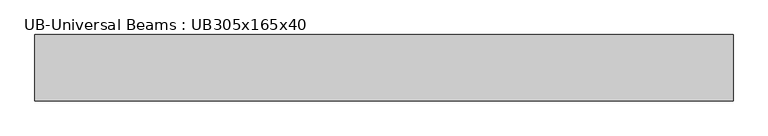
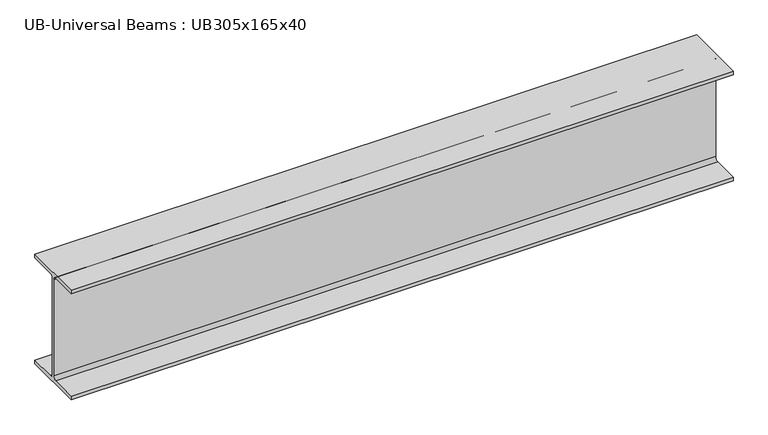
"""IFC4 building model written with IfcOpenShell, lengths in millimetres: beam geometry, UB-Universal Beams : UB305x165x40."""

from ifc_helpers import new_model, si_unit, point, frame, frame_2d, origin, place, context, project, spatial, polyline, circle_curve, trimmed, segment, composite_curve, outline, extrude, source, transform, mapped, element, save


def ub_universal_beams_ub305x165x40_86e0045c(model_context):
    return source(origin(), model_context, "Body", "SweptSolid", [
        extrude(outline(composite_curve([segment(polyline([(82.5, -141.5), (82.5, -151.7), (-82.5, -151.7), (-82.5, -141.5), (-11.9, -141.5)]), True, "CONTINUOUS"), segment(trimmed(circle_curve(frame_2d((-11.9, -132.6)), 8.9), [point((-11.9, -141.5))], [point((-3.0, -132.6))], True, "CARTESIAN"), True, "CONTINUOUS"), segment(polyline([(-3.0, -132.6), (-3.0, 132.6)]), True, "CONTINUOUS"), segment(trimmed(circle_curve(frame_2d((-11.9, 132.6)), 8.9), [point((-3.0, 132.6))], [point((-11.9, 141.5))], True, "CARTESIAN"), True, "CONTINUOUS"), segment(polyline([(-11.9, 141.5), (-82.5, 141.5), (-82.5, 151.7), (82.5, 151.7), (82.5, 141.5), (11.9, 141.5)]), True, "CONTINUOUS"), segment(trimmed(circle_curve(frame_2d((11.9, 132.6)), 8.9), [point((11.9, 141.5))], [point((3.0, 132.6))], True, "CARTESIAN"), True, "CONTINUOUS"), segment(polyline([(3.0, 132.6), (3.0, -132.6)]), True, "CONTINUOUS"), segment(trimmed(circle_curve(frame_2d((11.9, -132.6)), 8.9), [point((3.0, -132.6))], [point((11.9, -141.5))], True, "CARTESIAN"), True, "CONTINUOUS"), segment(polyline([(11.9, -141.5), (82.5, -141.5)]), True, "CONTINUOUS")], self_intersect=False)), frame((-877.25, 0.0, 0.0), z_axis=(1.0, 0.0, 0.0), x_axis=(0.0, 1.0, 0.0)), (0.0, 0.0, 1.0), 1732.3),
    ])


if __name__ == "__main__":
    model = new_model("IFC4")
    model_context = context("Model", 3, world=origin())
    ifc_project = project(units=[si_unit("LENGTHUNIT", "METRE", prefix="MILLI")], contexts=[model_context])
    site = spatial("IfcSite", under=ifc_project)
    building = spatial("IfcBuilding", under=site)
    placement = place(None, origin())
    ub_universal_beams_ub305x165x40_shape = ub_universal_beams_ub305x165x40_86e0045c(model_context)
    element("IfcBeam", 1, ObjectType="UB-Universal Beams : UB305x165x40", at=placement, inside=building, context=model_context, shape_type="MappedRepresentation", body=[
        mapped(ub_universal_beams_ub305x165x40_shape, transform((0.0, 0.0, 0.0), x_axis=(1.0, 0.0, 0.0), y_axis=(0.0, 1.0, 0.0), z_axis=(0.0, 0.0, 1.0))),
    ])
    save(model, "model.ifc")

# Revit data of these elements
# Type "UB-Universal Beams : UB305x165x40"
#   Section Name Key = "UB305X165X40"
#   Width = 16.5 cm
#   Web Thickness = 0.6 cm
#   Web Fillet = 0.89 cm
#   Warping Constant = 164000.0 cm⁶
#   Torsional Moment of Inertia = 14.70 cm⁴
#   Section Area = 51.3 cm²
#   Plastic Modulus weak axis = 142.0 cm³
#   Plastic Modulus strong axis = 623.0 cm³
#   Nominal Weight = 40.2999 kgf/m
#   Moment of Inertia weak axis = 764.00 cm⁴
#   Moment of Inertia strong axis = 8503.00 cm⁴
#   Height = 30.34 cm
#   Flange Thickness = 1.02 cm
#   Elastic Modulus weak axis = 92.6 cm³
#   Elastic Modulus strong axis = 560.0 cm³
#   Centroid Vertical = 15.17 cm
#   Centroid Horizontal = 8.25 cm
#   Bolt Spacing = 9.0 cm
#   Length [instance default] = 1500 mm
#   Structural Material [instance default] = Metal - Steel 43-275
#   Type Comments = ""
#   Assembly Code = ""
# Element 1 (IfcBeam, "UB-Universal Beams : UB305x165x40")
#   Materials on its faces: "Metal - Steel 43-275"
# Materials
#   "Metal - Steel 43-275": class "Metal", colour RGB 247 247 247, transparency 0, Cost = 0
